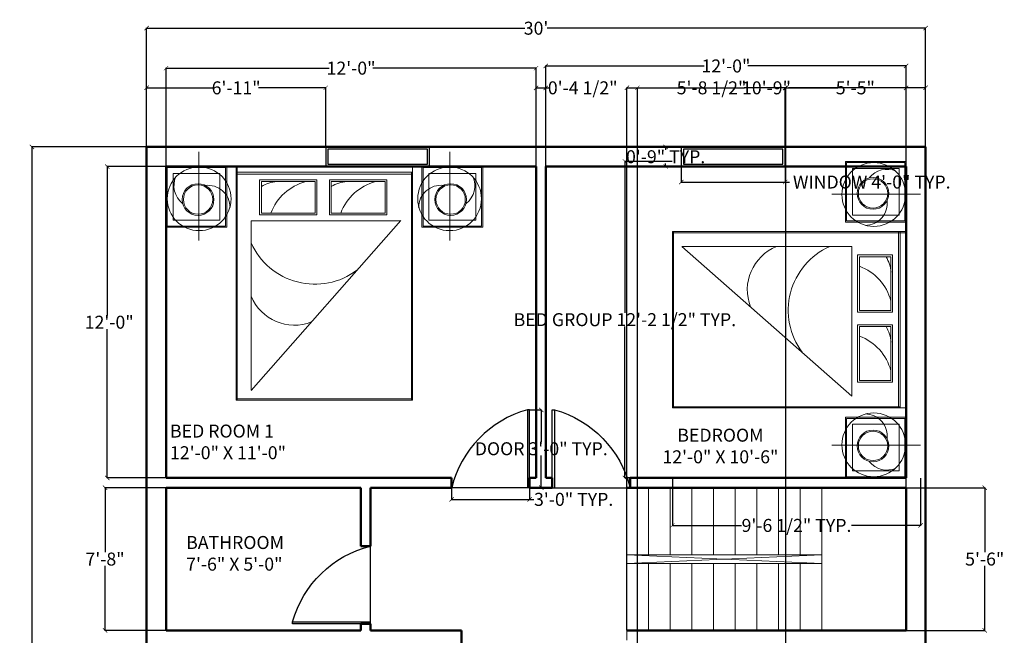
# Model space of a CAD drawing. Units: inches. Extents: x -40 to 418, y 1212 to 1787.
# Tile 3 of 3: x -40 to 415, y 1503 to 1787. Entities that reach past the tile are written whole.
import ezdxf

# ---------------------------------------------------------------- set-up
doc = ezdxf.new("R2010")
doc.units = ezdxf.units.IN
doc.header["$MEASUREMENT"] = 0
for name, color, linetype, lineweight in [('A-ANNO-DIMS', 2, 'Continuous', 18), ('A-AREA-IDEN', 7, 'Continuous', 25), ('A-DOOR', 4, 'Continuous', 25), ('A-FLOR-STRS', 7, 'Continuous', 18), ('A-FURN', 8, 'Continuous', 18), ('A-GLAZ', 4, 'Continuous', 25), ('A-WALL', 7, 'Continuous', 50)]:
    doc.layers.add(name, color=color, linetype=linetype, lineweight=lineweight)
doc.styles.get("Standard").update_dxf_attribs({"font": 'arial.ttf'})
doc.dimstyles.get("Standard").update_dxf_attribs({"dimtxt": 6, "dimasz": 2, "dimexe": 0.18, "dimexo": 0.0625, "dimgap": 0.09, "dimtad": 0, "dimtih": 1, "dimtoh": 1, "dimdec": 0, "dimzin": 0, "dimdsep": 46, "dimlunit": 4, "dimtxsty": 'Standard', "dimblk": 'ARCHTICK', "dimcen": 0.09, "dimadec": 0, "dimazin": 0, "dimtfac": 1, "dimtdec": 0, "dimtofl": 0, "dimtmove": 0, "dimatfit": 3, "dimldrblk": 'ARCHTICK', "dimfxl": 1, "dimtolj": 1, "dimtzin": 0, "dimarcsym": 0})

# ---------------------------------------------------------------- blocks, each defined once
blk = doc.blocks.new('_ArchTick')
at = {"color": 0, "linetype": 'ByBlock', "const_width": 0.15}
blk.add_lwpolyline([(-0.5, -0.5), (0.5, 0.5)], dxfattribs=at)
blk = doc.blocks.new('*D2')
at = {"layer": 'A-ANNO-DIMS', "color": 0, "lineweight": -2, "transparency": 16777216}
for p, q in [((27.43, 1719.7), (27.43, 1765.27)), ((27.43, 1765.09), (102.82, 1765.09)), ((198.43, 1765.09), (123.05, 1765.09)), ((198.43, 1719.7), (198.43, 1765.27))]:
    blk.add_line(p, q, dxfattribs=at)
at = {"layer": 'Defpoints', "color": 0, "transparency": 16777216}
for p in [(198.43, 1765.09), (27.43, 1719.64), (198.43, 1719.64)]:
    blk.add_point(p, dxfattribs=at)
at = {"layer": 'A-ANNO-DIMS', "color": 0, "lineweight": -2, "transparency": 16777216, "xscale": 2, "yscale": 2, "zscale": 2, "rotation": 180}
blk.add_blockref('_ArchTick', (27.43, 1765.09), dxfattribs=at)
at = {"layer": 'A-ANNO-DIMS', "color": 0, "lineweight": -2, "transparency": 16777216, "xscale": 2, "yscale": 2, "zscale": 2}
blk.add_blockref('_ArchTick', (198.43, 1765.09), dxfattribs=at)
at = {"layer": 'A-ANNO-DIMS', "color": 0, "transparency": 16777216, "insert": (112.93, 1765.09), "char_height": 6, "attachment_point": 5}
blk.add_mtext('\\A1;12\'-0"', dxfattribs=at)
blk = doc.blocks.new('*D3')
at = {"layer": 'A-ANNO-DIMS', "color": 0, "lineweight": -2, "transparency": 16777216}
for p, q in [((202.93, 1719.7), (202.93, 1766.27)), ((202.93, 1766.09), (276.07, 1766.09)), ((369.43, 1766.09), (296.3, 1766.09)), ((369.43, 1719.7), (369.43, 1766.27))]:
    blk.add_line(p, q, dxfattribs=at)
at = {"layer": 'Defpoints', "color": 0, "transparency": 16777216}
for p in [(369.43, 1766.09), (202.93, 1719.64), (369.43, 1719.64)]:
    blk.add_point(p, dxfattribs=at)
at = {"layer": 'A-ANNO-DIMS', "color": 0, "lineweight": -2, "transparency": 16777216, "xscale": 2, "yscale": 2, "zscale": 2, "rotation": 180}
blk.add_blockref('_ArchTick', (202.93, 1766.09), dxfattribs=at)
at = {"layer": 'A-ANNO-DIMS', "color": 0, "lineweight": -2, "transparency": 16777216, "xscale": 2, "yscale": 2, "zscale": 2}
blk.add_blockref('_ArchTick', (369.43, 1766.09), dxfattribs=at)
at = {"layer": 'A-ANNO-DIMS', "color": 0, "transparency": 16777216, "insert": (286.18, 1766.09), "char_height": 6, "attachment_point": 5}
blk.add_mtext('\\A1;12\'-0"', dxfattribs=at)
blk = doc.blocks.new('*D4')
at = {"layer": 'A-ANNO-DIMS', "color": 0, "lineweight": -2, "transparency": 16777216}
for p, q in [((18.43, 1728.7), (18.43, 1783.74)), ((378.43, 1728.7), (378.43, 1783.74)), ((18.43, 1783.56), (193.26, 1783.56)), ((378.43, 1783.56), (203.61, 1783.56))]:
    blk.add_line(p, q, dxfattribs=at)
at = {"layer": 'Defpoints', "color": 0, "transparency": 16777216}
for p in [(378.43, 1783.56), (18.43, 1728.64), (378.43, 1728.64)]:
    blk.add_point(p, dxfattribs=at)
at = {"layer": 'A-ANNO-DIMS', "color": 0, "lineweight": -2, "transparency": 16777216, "xscale": 2, "yscale": 2, "zscale": 2, "rotation": 180}
blk.add_blockref('_ArchTick', (18.43, 1783.56), dxfattribs=at)
at = {"layer": 'A-ANNO-DIMS', "color": 0, "lineweight": -2, "transparency": 16777216, "xscale": 2, "yscale": 2, "zscale": 2}
blk.add_blockref('_ArchTick', (378.43, 1783.56), dxfattribs=at)
at = {"layer": 'A-ANNO-DIMS', "color": 0, "transparency": 16777216, "insert": (198.43, 1783.56), "char_height": 6, "attachment_point": 5}
blk.add_mtext("\\A1;30'", dxfattribs=at)
blk = doc.blocks.new('*D5')
at = {"layer": 'A-ANNO-DIMS', "color": 0, "lineweight": -2, "transparency": 16777216}
for p, q in [((18.37, 1728.64), (-34.7, 1728.64)), ((-34.52, 1728.64), (-34.52, 1491.79)), ((-34.52, 1248.64), (-34.52, 1485.48)), ((18.37, 1248.64), (-34.7, 1248.64))]:
    blk.add_line(p, q, dxfattribs=at)
at = {"layer": 'Defpoints', "color": 0, "transparency": 16777216}
for p in [(-34.52, 1728.64), (18.43, 1728.64), (18.43, 1248.64)]:
    blk.add_point(p, dxfattribs=at)
at = {"layer": 'A-ANNO-DIMS', "color": 0, "lineweight": -2, "transparency": 16777216, "xscale": 2, "yscale": 2, "zscale": 2}
for p, rotation in [((-34.52, 1728.64), 90), ((-34.52, 1248.64), 270)]:
    blk.add_blockref('_ArchTick', p, dxfattribs=dict(at, rotation=rotation))
at = {"layer": 'A-ANNO-DIMS', "color": 0, "transparency": 16777216, "insert": (-34.52, 1488.64), "char_height": 6, "attachment_point": 5}
blk.add_mtext("\\A1;40'", dxfattribs=at)
blk = doc.blocks.new('*D6')
at = {"layer": 'A-ANNO-DIMS', "color": 0, "lineweight": -2, "transparency": 16777216}
for p, q in [((27.37, 1719.64), (0.07, 1719.64)), ((0.25, 1719.64), (0.25, 1650.79)), ((0.25, 1575.64), (0.25, 1644.48)), ((27.37, 1575.64), (0.07, 1575.64))]:
    blk.add_line(p, q, dxfattribs=at)
at = {"layer": 'Defpoints', "color": 0, "transparency": 16777216}
for p in [(0.25, 1719.64), (27.43, 1719.64), (27.43, 1575.64)]:
    blk.add_point(p, dxfattribs=at)
at = {"layer": 'A-ANNO-DIMS', "color": 0, "lineweight": -2, "transparency": 16777216, "xscale": 2, "yscale": 2, "zscale": 2}
for p, rotation in [((0.25, 1719.64), 90), ((0.25, 1575.64), 270)]:
    blk.add_blockref('_ArchTick', p, dxfattribs=dict(at, rotation=rotation))
at = {"layer": 'A-ANNO-DIMS', "color": 0, "transparency": 16777216, "insert": (0.25, 1647.64), "char_height": 6, "attachment_point": 5}
blk.add_mtext('\\A1; 12\'-0"', dxfattribs=at)
blk = doc.blocks.new('*D7')
at = {"layer": 'A-ANNO-DIMS', "color": 0, "lineweight": -2, "transparency": 16777216}
for p, q in [((27.37, 1571.14), (-0.93, 1571.14)), ((-0.75, 1571.14), (-0.75, 1541.29)), ((-0.75, 1505.14), (-0.75, 1534.98)), ((27.37, 1505.14), (-0.93, 1505.14))]:
    blk.add_line(p, q, dxfattribs=at)
at = {"layer": 'Defpoints', "color": 0, "transparency": 16777216}
for p in [(-0.75, 1571.14), (27.43, 1571.14), (27.43, 1505.14)]:
    blk.add_point(p, dxfattribs=at)
at = {"layer": 'A-ANNO-DIMS', "color": 0, "lineweight": -2, "transparency": 16777216, "xscale": 2, "yscale": 2, "zscale": 2}
for p, rotation in [((-0.75, 1571.14), 90), ((-0.75, 1505.14), 270)]:
    blk.add_blockref('_ArchTick', p, dxfattribs=dict(at, rotation=rotation))
at = {"layer": 'A-ANNO-DIMS', "color": 0, "transparency": 16777216, "insert": (-0.75, 1538.14), "char_height": 6, "attachment_point": 5}
blk.add_mtext('\\A1;7\'-8"', dxfattribs=at)
blk = doc.blocks.new('DESDFGHJUI')
for p, q in [((-198.91, 1688.99), (-198.91, 1729.95)), ((-82.83, 1688.99), (-82.83, 1729.95)), ((-214.04, 1695.16), (-214.04, 1723.24)), ((-214.04, 1723.24), (-185.96, 1723.24)), ((-213.5, 1695.7), (-213.5, 1722.7)), ((-213.5, 1722.7), (-186.5, 1722.7)), ((-210.8, 1698.4), (-210.8, 1720)), ((-210.8, 1720), (-189.2, 1720)), ((-189.2, 1720), (-189.2, 1698.4)), ((-186.5, 1722.7), (-186.5, 1695.7)), ((-185.96, 1723.24), (-185.96, 1695.16)), ((-181.64, 1723.24), (-181.64, 1615.24)), ((-181.64, 1723.24), (-100.1, 1723.24)), ((-181.64, 1720.54), (-100.1, 1720.54)), ((-181.1, 1723.24), (-181.1, 1615.24)), ((-100.64, 1720.54), (-100.64, 1615.24)), ((-100.1, 1723.24), (-100.1, 1615.24)), ((-67.7, 1723.24), (-95.78, 1723.24)), ((-95.78, 1723.24), (-95.78, 1695.16)), ((-68.24, 1722.7), (-95.24, 1722.7)), ((-95.24, 1722.7), (-95.24, 1695.7)), ((-70.94, 1720), (-92.54, 1720)), ((-92.54, 1720), (-92.54, 1698.4)), ((-70.94, 1698.4), (-70.94, 1720)), ((-68.24, 1695.7), (-68.24, 1722.7)), ((-67.7, 1695.16), (-67.7, 1723.24)), ((-181.64, 1719.73), (-100.1, 1719.73)), ((-170.78, 1700.83), (-170.78, 1717.03)), ((-170.78, 1717.03), (-144.32, 1717.03)), ((-169.97, 1701.64), (-169.97, 1716.22)), ((-169.97, 1716.22), (-145.13, 1716.22)), ((-145.13, 1716.22), (-145.13, 1701.64)), ((-144.32, 1717.03), (-144.32, 1700.83)), ((-138.48, 1700.83), (-138.48, 1717.03)), ((-138.48, 1717.03), (-112.02, 1717.03)), ((-137.67, 1701.64), (-137.67, 1716.22)), ((-137.67, 1716.22), (-112.83, 1716.22)), ((-112.83, 1716.22), (-112.83, 1701.64)), ((-112.02, 1717.03), (-112.02, 1700.83)), ((-189.2, 1698.4), (-210.8, 1698.4)), ((-174.68, 1619.61), (-105.47, 1698.21)), ((-174.64, 1619.8), (-174.64, 1698.13)), ((-174.64, 1698.13), (-105.54, 1698.13)), ((-170.78, 1700.83), (-144.32, 1700.83)), ((-169.97, 1701.64), (-145.13, 1701.64)), ((-138.48, 1700.83), (-112.02, 1700.83)), ((-137.67, 1701.64), (-112.83, 1701.64)), ((-92.54, 1698.4), (-70.94, 1698.4)), ((-185.96, 1695.16), (-214.04, 1695.16)), ((-186.5, 1695.7), (-213.5, 1695.7)), ((-95.78, 1695.16), (-67.7, 1695.16)), ((-95.24, 1695.7), (-68.24, 1695.7)), ((-131.52, 1615.74), (-181.64, 1615.74)), ((-100.1, 1615.78), (-175.16, 1615.78)), ((-100.1, 1615.24), (-181.64, 1615.24))]:
    blk.add_line(p, q)
for centre, radius in [((-198.74, 1708.29), 14.73), ((-83.01, 1708.29), 14.73), ((-199.23, 1707.96), 7.32), ((-199.23, 1707.96), 6.78), ((-82.52, 1707.96), 7.32), ((-82.52, 1707.96), 6.78)]:
    blk.add_circle(centre, radius)
for centre, radius, start, end in [((-200.04, 1714.33), 10.36, 155.9567, 231.7564), ((-161.57, 1700.2), 16.13, 94.4656, 121.4122), ((-143.54, 1693.44), 23.54, 104.6626, 159.6122), ((-129.26, 1700.2), 16.13, 94.4656, 121.4122), ((-111.24, 1693.44), 23.54, 104.6626, 159.6122), ((-81.71, 1714.33), 10.36, 308.2436, 24.0433), ((-194.74, 1704.25), 10.3, 0.4104, 96.764), ((-87.01, 1704.25), 10.3, 83.236, 179.5896), ((-145.2, 1701.08), 32.28, 204.0563, 306.8492), ((-154.7, 1671.44), 21.57, 202.1275, 291.5505)]:
    blk.add_arc(centre, radius, start, end)
blk = doc.blocks.new('EREGTHYGUI')
for p, q in [((195.43, 1607.14), (194.43, 1607.14)), ((194.43, 1607.14), (194.43, 1571.14)), ((195.43, 1571.14), (195.43, 1607.14)), ((195.43, 1571.14), (159.43, 1571.14))]:
    blk.add_line(p, q)
blk.add_arc((207.79, 1559.14), 49.82, 105.5486, 166.0653)
blk = doc.blocks.new('WIN-48IN')
for points in [[(0, 0), (9, 0), (9, 48), (0, 48)], [(1, 1), (8, 1), (8, 47), (1, 47)]]:
    blk.add_lwpolyline(points, close=True)
blk = doc.blocks.new('*D17')
at = {"layer": 'A-ANNO-DIMS', "color": 0, "lineweight": -2, "transparency": 16777216}
for p, q in [((195.5, 1607.14), (201.01, 1607.14)), ((200.83, 1607.14), (200.83, 1592.33)), ((200.83, 1571.14), (200.83, 1585.94)), ((195.5, 1571.14), (201.01, 1571.14))]:
    blk.add_line(p, q, dxfattribs=at)
at = {"layer": 'Defpoints', "color": 0, "transparency": 16777216}
for p in [(195.43, 1607.14), (200.83, 1607.14), (195.43, 1571.14)]:
    blk.add_point(p, dxfattribs=at)
at = {"layer": 'A-ANNO-DIMS', "color": 0, "lineweight": -2, "transparency": 16777216, "xscale": 2, "yscale": 2, "zscale": 2}
for p, rotation in [((200.83, 1607.14), 90), ((200.83, 1571.14), 270)]:
    blk.add_blockref('_ArchTick', p, dxfattribs=dict(at, rotation=rotation))
at = {"layer": 'A-ANNO-DIMS', "color": 0, "transparency": 16777216, "insert": (200.83, 1589.14), "char_height": 6, "attachment_point": 5}
blk.add_mtext('\\A1;DOOR 3\'-0" TYP.', dxfattribs=at)
blk = doc.blocks.new('*D18')
at = {"layer": 'A-ANNO-DIMS', "color": 0, "lineweight": -2, "transparency": 16777216}
for p, q in [((159.43, 1571.07), (159.43, 1565.56)), ((195.43, 1571.07), (195.43, 1565.56)), ((159.43, 1565.74), (195.43, 1565.74)), ((195.43, 1565.74), (197.43, 1565.74))]:
    blk.add_line(p, q, dxfattribs=at)
at = {"layer": 'Defpoints', "color": 0, "transparency": 16777216}
for p in [(159.43, 1571.14), (195.43, 1571.14), (195.43, 1565.74)]:
    blk.add_point(p, dxfattribs=at)
at = {"layer": 'A-ANNO-DIMS', "color": 0, "lineweight": -2, "transparency": 16777216, "xscale": 2, "yscale": 2, "zscale": 2, "rotation": 180}
blk.add_blockref('_ArchTick', (159.43, 1565.74), dxfattribs=at)
at = {"layer": 'A-ANNO-DIMS', "color": 0, "lineweight": -2, "transparency": 16777216, "xscale": 2, "yscale": 2, "zscale": 2}
blk.add_blockref('_ArchTick', (195.43, 1565.74), dxfattribs=at)
at = {"layer": 'A-ANNO-DIMS', "color": 0, "transparency": 16777216, "insert": (215.81, 1565.74), "char_height": 6, "attachment_point": 5}
blk.add_mtext('\\A1;3\'-0" TYP.', dxfattribs=at)
blk = doc.blocks.new('*D19')
at = {"layer": 'A-ANNO-DIMS', "color": 0, "lineweight": -2, "transparency": 16777216}
for p, q in [((265.52, 1719.57), (265.52, 1712.26)), ((313.52, 1719.57), (313.52, 1712.26)), ((265.52, 1712.44), (313.52, 1712.44)), ((313.52, 1712.44), (315.52, 1712.44))]:
    blk.add_line(p, q, dxfattribs=at)
at = {"layer": 'Defpoints', "color": 0, "transparency": 16777216}
for p in [(265.52, 1719.64), (313.52, 1719.64), (313.52, 1712.44)]:
    blk.add_point(p, dxfattribs=at)
at = {"layer": 'A-ANNO-DIMS', "color": 0, "lineweight": -2, "transparency": 16777216, "xscale": 2, "yscale": 2, "zscale": 2, "rotation": 180}
blk.add_blockref('_ArchTick', (265.52, 1712.44), dxfattribs=at)
at = {"layer": 'A-ANNO-DIMS', "color": 0, "lineweight": -2, "transparency": 16777216, "xscale": 2, "yscale": 2, "zscale": 2}
blk.add_blockref('_ArchTick', (313.52, 1712.44), dxfattribs=at)
at = {"layer": 'A-ANNO-DIMS', "color": 0, "transparency": 16777216, "insert": (353.57, 1712.44), "char_height": 6, "attachment_point": 5}
blk.add_mtext('\\A1;WINDOW 4\'-0" TYP.', dxfattribs=at)
blk = doc.blocks.new('*D20')
at = {"layer": 'A-ANNO-DIMS', "color": 0, "lineweight": -2, "transparency": 16777216}
for p, q in [((265.46, 1728.64), (258.14, 1728.64)), ((258.32, 1728.64), (258.32, 1727.29)), ((258.32, 1719.64), (258.32, 1720.98)), ((265.46, 1719.64), (258.14, 1719.64))]:
    blk.add_line(p, q, dxfattribs=at)
at = {"layer": 'Defpoints', "color": 0, "transparency": 16777216}
for p in [(265.52, 1728.64), (258.32, 1719.64), (265.52, 1719.64)]:
    blk.add_point(p, dxfattribs=at)
at = {"layer": 'A-ANNO-DIMS', "color": 0, "lineweight": -2, "transparency": 16777216, "xscale": 2, "yscale": 2, "zscale": 2}
for p, rotation in [((258.32, 1728.64), 90), ((258.32, 1719.64), 270)]:
    blk.add_blockref('_ArchTick', p, dxfattribs=dict(at, rotation=rotation))
at = {"layer": 'A-ANNO-DIMS', "color": 0, "transparency": 16777216, "insert": (258.32, 1724.14), "char_height": 6, "attachment_point": 5}
blk.add_mtext('\\A1;0\'-9" TYP.', dxfattribs=at)
blk = doc.blocks.new('*D23')
at = {"layer": 'A-ANNO-DIMS', "color": 0, "lineweight": -2, "transparency": 16777216}
for p, q in [((261.37, 1721.98), (239.3, 1721.98)), ((239.48, 1721.98), (239.48, 1652)), ((239.48, 1575.64), (239.48, 1645.61)), ((261.37, 1575.64), (239.3, 1575.64))]:
    blk.add_line(p, q, dxfattribs=at)
at = {"layer": 'Defpoints', "color": 0, "transparency": 16777216}
for p in [(261.43, 1721.98), (239.48, 1575.64), (261.43, 1575.64)]:
    blk.add_point(p, dxfattribs=at)
at = {"layer": 'A-ANNO-DIMS', "color": 0, "lineweight": -2, "transparency": 16777216, "xscale": 2, "yscale": 2, "zscale": 2}
for p, rotation in [((239.48, 1721.98), 90), ((239.48, 1575.64), 270)]:
    blk.add_blockref('_ArchTick', p, dxfattribs=dict(at, rotation=rotation))
at = {"layer": 'A-ANNO-DIMS', "color": 0, "transparency": 16777216, "insert": (239.48, 1648.81), "char_height": 6, "attachment_point": 5}
blk.add_mtext('\\A1;BED GROUP 12\'-2 1/2" TYP.', dxfattribs=at)
blk = doc.blocks.new('*D24')
at = {"layer": 'A-ANNO-DIMS', "color": 0, "lineweight": -2, "transparency": 16777216}
for p, q in [((261.43, 1575.57), (261.43, 1553.51)), ((376.15, 1575.57), (376.15, 1553.51)), ((261.43, 1553.69), (293.42, 1553.69)), ((376.15, 1553.69), (344.16, 1553.69))]:
    blk.add_line(p, q, dxfattribs=at)
at = {"layer": 'Defpoints', "color": 0, "transparency": 16777216}
for p in [(261.43, 1575.64), (376.15, 1575.64), (376.15, 1553.69)]:
    blk.add_point(p, dxfattribs=at)
at = {"layer": 'A-ANNO-DIMS', "color": 0, "lineweight": -2, "transparency": 16777216, "xscale": 2, "yscale": 2, "zscale": 2, "rotation": 180}
blk.add_blockref('_ArchTick', (261.43, 1553.69), dxfattribs=at)
at = {"layer": 'A-ANNO-DIMS', "color": 0, "lineweight": -2, "transparency": 16777216, "xscale": 2, "yscale": 2, "zscale": 2}
blk.add_blockref('_ArchTick', (376.15, 1553.69), dxfattribs=at)
at = {"layer": 'A-ANNO-DIMS', "color": 0, "transparency": 16777216, "insert": (318.79, 1553.69), "char_height": 6, "attachment_point": 5}
blk.add_mtext('\\A1;9\'-6 1/2" TYP.', dxfattribs=at)
blk = doc.blocks.new('*D31')
at = {"layer": 'A-ANNO-DIMS', "color": 0, "lineweight": -2, "transparency": 16777216}
for p, q in [((240.43, 1505.2), (240.43, 1756.17)), ((240.43, 1755.99), (294.82, 1755.99)), ((369.43, 1755.99), (315.05, 1755.99)), ((369.43, 1505.2), (369.43, 1756.17))]:
    blk.add_line(p, q, dxfattribs=at)
at = {"layer": 'Defpoints', "color": 0, "transparency": 16777216}
for p in [(369.43, 1755.99), (240.43, 1505.14), (369.43, 1505.14)]:
    blk.add_point(p, dxfattribs=at)
at = {"layer": 'A-ANNO-DIMS', "color": 0, "lineweight": -2, "transparency": 16777216, "xscale": 2, "yscale": 2, "zscale": 2, "rotation": 180}
blk.add_blockref('_ArchTick', (240.43, 1755.99), dxfattribs=at)
at = {"layer": 'A-ANNO-DIMS', "color": 0, "lineweight": -2, "transparency": 16777216, "xscale": 2, "yscale": 2, "zscale": 2}
blk.add_blockref('_ArchTick', (369.43, 1755.99), dxfattribs=at)
at = {"layer": 'A-ANNO-DIMS', "color": 0, "transparency": 16777216, "insert": (304.93, 1755.99), "char_height": 6, "attachment_point": 5}
blk.add_mtext('\\A1;10\'-9"', dxfattribs=at)
blk = doc.blocks.new('*D32')
at = {"layer": 'A-ANNO-DIMS', "color": 0, "lineweight": -2, "transparency": 16777216}
for p, q in [((369.5, 1571.14), (405.96, 1571.14)), ((405.78, 1571.14), (405.78, 1541.29)), ((405.78, 1505.14), (405.78, 1534.98)), ((369.5, 1505.14), (405.96, 1505.14))]:
    blk.add_line(p, q, dxfattribs=at)
at = {"layer": 'Defpoints', "color": 0, "transparency": 16777216}
for p in [(369.43, 1571.14), (405.78, 1571.14), (369.43, 1505.14)]:
    blk.add_point(p, dxfattribs=at)
at = {"layer": 'A-ANNO-DIMS', "color": 0, "lineweight": -2, "transparency": 16777216, "xscale": 2, "yscale": 2, "zscale": 2}
for p, rotation in [((405.78, 1571.14), 90), ((405.78, 1505.14), 270)]:
    blk.add_blockref('_ArchTick', p, dxfattribs=dict(at, rotation=rotation))
at = {"layer": 'A-ANNO-DIMS', "color": 0, "transparency": 16777216, "insert": (405.78, 1538.14), "char_height": 6, "attachment_point": 5}
blk.add_mtext('\\A1;5\'-6"', dxfattribs=at)
blk = doc.blocks.new('*D36')
at = {"layer": 'A-ANNO-DIMS', "color": 0, "lineweight": -2, "transparency": 16777216}
for p, q in [((18.43, 1728.7), (18.43, 1756.17)), ((18.43, 1755.99), (49.41, 1755.99)), ((101.22, 1755.99), (70.24, 1755.99)), ((101.22, 1728.7), (101.22, 1756.17))]:
    blk.add_line(p, q, dxfattribs=at)
at = {"layer": 'Defpoints', "color": 0, "transparency": 16777216}
for p in [(101.22, 1755.99), (18.43, 1728.64), (101.22, 1728.64)]:
    blk.add_point(p, dxfattribs=at)
at = {"layer": 'A-ANNO-DIMS', "color": 0, "lineweight": -2, "transparency": 16777216, "xscale": 2, "yscale": 2, "zscale": 2, "rotation": 180}
blk.add_blockref('_ArchTick', (18.43, 1755.99), dxfattribs=at)
at = {"layer": 'A-ANNO-DIMS', "color": 0, "lineweight": -2, "transparency": 16777216, "xscale": 2, "yscale": 2, "zscale": 2}
blk.add_blockref('_ArchTick', (101.22, 1755.99), dxfattribs=at)
at = {"layer": 'A-ANNO-DIMS', "color": 0, "transparency": 16777216, "insert": (59.83, 1755.99), "char_height": 6, "attachment_point": 5}
blk.add_mtext('\\A1;6\'-11"', dxfattribs=at)
blk = doc.blocks.new('*D37')
at = {"layer": 'A-ANNO-DIMS', "color": 0, "lineweight": -2, "transparency": 16777216}
for p, q in [((313.52, 1728.7), (313.52, 1756.17)), ((313.52, 1755.99), (337.91, 1755.99)), ((378.43, 1755.99), (354.04, 1755.99)), ((378.43, 1728.7), (378.43, 1756.17))]:
    blk.add_line(p, q, dxfattribs=at)
at = {"layer": 'Defpoints', "color": 0, "transparency": 16777216}
for p in [(378.43, 1755.99), (313.52, 1728.64), (378.43, 1728.64)]:
    blk.add_point(p, dxfattribs=at)
at = {"layer": 'A-ANNO-DIMS', "color": 0, "lineweight": -2, "transparency": 16777216, "xscale": 2, "yscale": 2, "zscale": 2, "rotation": 180}
blk.add_blockref('_ArchTick', (313.52, 1755.99), dxfattribs=at)
at = {"layer": 'A-ANNO-DIMS', "color": 0, "lineweight": -2, "transparency": 16777216, "xscale": 2, "yscale": 2, "zscale": 2}
blk.add_blockref('_ArchTick', (378.43, 1755.99), dxfattribs=at)
at = {"layer": 'A-ANNO-DIMS', "color": 0, "transparency": 16777216, "insert": (345.98, 1755.99), "char_height": 6, "attachment_point": 5}
blk.add_mtext('\\A1;5\'-5"', dxfattribs=at)
blk = doc.blocks.new('*D39')
at = {"layer": 'A-ANNO-DIMS', "color": 0, "lineweight": -2, "transparency": 16777216}
for p, q in [((245.24, 1474.1), (245.24, 1756.17)), ((245.24, 1755.99), (264.49, 1755.99)), ((313.85, 1755.99), (294.6, 1755.99)), ((313.85, 1474.1), (313.85, 1756.17))]:
    blk.add_line(p, q, dxfattribs=at)
at = {"layer": 'Defpoints', "color": 0, "transparency": 16777216}
for p in [(313.85, 1755.99), (245.24, 1474.03), (313.85, 1474.03)]:
    blk.add_point(p, dxfattribs=at)
at = {"layer": 'A-ANNO-DIMS', "color": 0, "lineweight": -2, "transparency": 16777216, "xscale": 2, "yscale": 2, "zscale": 2, "rotation": 180}
blk.add_blockref('_ArchTick', (245.24, 1755.99), dxfattribs=at)
at = {"layer": 'A-ANNO-DIMS', "color": 0, "lineweight": -2, "transparency": 16777216, "xscale": 2, "yscale": 2, "zscale": 2}
blk.add_blockref('_ArchTick', (313.85, 1755.99), dxfattribs=at)
at = {"layer": 'A-ANNO-DIMS', "color": 0, "transparency": 16777216, "insert": (279.54, 1755.99), "char_height": 6, "attachment_point": 5}
blk.add_mtext('\\A1;5\'-8 1/2"', dxfattribs=at)
blk = doc.blocks.new('*D44')
at = {"layer": 'A-ANNO-DIMS', "color": 0, "lineweight": -2, "transparency": 16777216}
for p, q in [((198.43, 1719.7), (198.43, 1756.17)), ((198.43, 1755.99), (202.93, 1755.99)), ((202.93, 1719.7), (202.93, 1756.17)), ((202.93, 1755.99), (204.93, 1755.99))]:
    blk.add_line(p, q, dxfattribs=at)
at = {"layer": 'Defpoints', "color": 0, "transparency": 16777216}
for p in [(202.93, 1755.99), (198.43, 1719.64), (202.93, 1719.64)]:
    blk.add_point(p, dxfattribs=at)
at = {"layer": 'A-ANNO-DIMS', "color": 0, "lineweight": -2, "transparency": 16777216, "xscale": 2, "yscale": 2, "zscale": 2, "rotation": 180}
blk.add_blockref('_ArchTick', (198.43, 1755.99), dxfattribs=at)
at = {"layer": 'A-ANNO-DIMS', "color": 0, "lineweight": -2, "transparency": 16777216, "xscale": 2, "yscale": 2, "zscale": 2}
blk.add_blockref('_ArchTick', (202.93, 1755.99), dxfattribs=at)
at = {"layer": 'A-ANNO-DIMS', "color": 0, "transparency": 16777216, "insert": (219.99, 1755.99), "char_height": 6, "attachment_point": 5}
blk.add_mtext('\\A1;0\'-4 1/2"', dxfattribs=at)

msp = doc.modelspace()

# ---------------------------------------------------------------- linework, layer by layer
at = {"layer": 'A-FLOR-STRS'}
for p, q in [((240.43, 1571.14), (240.43, 1540.14)), ((250.43, 1571.14), (250.43, 1540.14)), ((260.43, 1571.14), (260.43, 1540.14)), ((270.43, 1571.14), (270.43, 1540.14)), ((280.43, 1571.14), (280.43, 1540.14)), ((290.43, 1571.14), (290.43, 1540.14)), ((300.43, 1571.14), (300.43, 1540.14)), ((310.43, 1571.14), (310.43, 1540.14)), ((320.43, 1571.14), (320.43, 1540.14)), ((330.43, 1571.14), (330.43, 1505.14)), ((330.43, 1540.14), (240.43, 1540.14)), ((240.43, 1536.14), (330.43, 1540.14)), ((240.43, 1540.14), (330.43, 1536.14)), ((330.43, 1536.14), (240.43, 1536.14)), ((240.43, 1536.14), (240.43, 1500.64)), ((250.43, 1536.14), (250.43, 1505.14)), ((260.43, 1536.14), (260.43, 1505.14)), ((270.43, 1536.14), (270.43, 1505.14)), ((280.43, 1536.14), (280.43, 1505.14)), ((290.43, 1536.14), (290.43, 1505.14)), ((300.43, 1536.14), (300.43, 1505.14)), ((310.43, 1536.14), (310.43, 1505.14)), ((320.43, 1536.14), (320.43, 1505.14))]:
    msp.add_line(p, q, dxfattribs=at)
at = {"layer": 'A-WALL'}
for p, q in [((18.43, 1728.64), (378.43, 1728.64)), ((18.43, 1248.64), (18.43, 1728.64)), ((378.43, 1728.64), (378.43, 1248.64)), ((27.43, 1719.64), (198.43, 1719.64)), ((27.43, 1575.64), (27.43, 1719.64)), ((198.43, 1719.64), (198.43, 1575.64)), ((202.93, 1719.64), (202.93, 1575.64)), ((202.93, 1719.64), (369.43, 1719.64)), ((369.43, 1719.64), (369.43, 1575.64)), ((27.43, 1575.64), (159.43, 1575.64)), ((159.43, 1575.64), (159.43, 1571.14)), ((195.43, 1575.64), (195.43, 1571.14)), ((195.43, 1575.64), (198.43, 1575.64)), ((202.93, 1575.64), (205.93, 1575.64)), ((205.93, 1575.64), (205.93, 1571.14)), ((241.93, 1575.64), (241.93, 1571.14)), ((241.93, 1575.64), (369.43, 1575.64)), ((27.43, 1571.14), (117.43, 1571.14)), ((27.43, 1505.14), (27.43, 1571.14)), ((117.43, 1544.14), (117.43, 1571.14)), ((121.93, 1571.14), (159.43, 1571.14)), ((121.93, 1544.14), (121.93, 1571.14)), ((195.43, 1571.14), (205.93, 1571.14)), ((240.43, 1571.14), (369.43, 1571.14)), ((369.43, 1571.14), (369.43, 1505.14)), ((117.43, 1544.14), (121.93, 1544.14)), ((117.43, 1505.14), (117.43, 1508.14)), ((117.43, 1508.14), (121.93, 1508.14)), ((121.93, 1505.14), (121.93, 1508.14)), ((27.43, 1505.14), (117.43, 1505.14)), ((121.93, 1505.14), (163.93, 1505.14)), ((163.93, 1443.64), (163.93, 1505.14)), ((240.43, 1505.14), (369.43, 1505.14))]:
    msp.add_line(p, q, dxfattribs=at)

# ---------------------------------------------------------------- block references
at = {"layer": 'A-DOOR'}
msp.add_blockref('EREGTHYGUI', (0, 0), dxfattribs=at)
at = {"layer": 'A-DOOR', "xscale": -1}
msp.add_blockref('EREGTHYGUI', (401.37, 0), dxfattribs=at)
at = {"layer": 'A-DOOR', "xscale": -1, "rotation": 90}
msp.add_blockref('EREGTHYGUI', (1693.07, 1703.57), dxfattribs=at)
at = {"layer": 'A-FURN'}
msp.add_blockref('DESDFGHJUI', (241.48, -3.6), dxfattribs=at)
at = {"layer": 'A-FURN', "rotation": 270}
msp.add_blockref('DESDFGHJUI', (-1353.8, 1507.93), dxfattribs=at)
at = {"layer": 'A-GLAZ', "rotation": 269.9999999999995}
for p in [(101.22, 1728.64), (265.52, 1728.64)]:
    msp.add_blockref('WIN-48IN', p, dxfattribs=at)

# ---------------------------------------------------------------- texts
at = {"layer": 'A-AREA-IDEN', "char_height": 6, "attachment_point": 1}
for s, width, insert in [(' BED ROOM 1\\P 12\'-0" X 11\'-0"', 120.8402, (27.43, 1600.31)), ('\\pxqc;BEDROOM\\P12\'-0" X 10\'-6"', 74.3114, (246.48, 1598.41)), ('BATHROOM\\P7\'-6" X 5\'-0"', 215.4125, (36.73, 1548.79))]:
    msp.add_mtext_dynamic_manual_height_columns(s, width=width, gutter_width=30, heights=[0], dxfattribs=dict(at, insert=insert))

# ---------------------------------------------------------------- dimensions: what is measured, and where the dimension line sits
at = {"layer": 'A-ANNO-DIMS'}
for base, p1, p2, override, picture, middle in [((378.43, 1783.56), (18.43, 1728.64), (378.43, 1728.64), {"dimclrd": 0, "dimclre": 0, "dimclrt": 0}, '*D4', (198.43, 1783.56)), ((202.93, 1755.99), (198.43, 1719.64), (202.93, 1719.64), {"dimdec": 1, "dimlfac": 1, "dimrnd": 0, "dimzin": 1, "dimdsep": 46, "dimlunit": 4, "dimfrac": 2}, '*D44', (219.99, 1755.99)), ((313.85, 1755.99), (245.24, 1474.03), (313.85, 1474.03), {"dimdec": 1, "dimlfac": 1, "dimrnd": 0, "dimzin": 1, "dimdsep": 46, "dimlunit": 4, "dimfrac": 2}, '*D39', (279.54, 1755.99)), ((101.22, 1755.99), (18.43, 1728.64), (101.22, 1728.64), {"dimdec": 1, "dimlfac": 1, "dimrnd": 0, "dimzin": 1, "dimdsep": 46, "dimlunit": 4, "dimfrac": 2}, '*D36', (59.83, 1755.99)), ((369.43, 1755.99), (240.43, 1505.14), (369.43, 1505.14), {"dimdec": 1, "dimlfac": 1, "dimrnd": 0, "dimzin": 1, "dimdsep": 46, "dimlunit": 4, "dimfrac": 2}, '*D31', (304.93, 1755.99)), ((378.43, 1755.99), (313.52, 1728.64), (378.43, 1728.64), {"dimdec": 1, "dimlfac": 1, "dimrnd": 0, "dimzin": 1, "dimdsep": 46, "dimlunit": 4, "dimfrac": 2}, '*D37', (345.98, 1755.99))]:
    dim = msp.add_linear_dim(base=base, p1=p1, p2=p2, dimstyle='Standard', override=override, dxfattribs=at)
    dim.commit()
    dim.dimension.update_dxf_attribs({"geometry": picture, "text_midpoint": middle})
for base, p1, p2, text, override, picture, middle in [((198.43, 1765.09), (27.43, 1719.64), (198.43, 1719.64), '12\'-0"', {"dimclrd": 0, "dimclre": 0, "dimclrt": 0}, '*D2', (112.93, 1765.09)), ((369.43, 1766.09), (202.93, 1719.64), (369.43, 1719.64), '12\'-0"', {"dimclrd": 0, "dimclre": 0, "dimclrt": 0}, '*D3', (286.18, 1766.09)), ((313.52, 1712.44), (265.52, 1719.64), (313.52, 1719.64), 'WINDOW <> TYP.', {"dimdec": 1, "dimlfac": 1, "dimrnd": 0, "dimzin": 1, "dimdsep": 46, "dimlunit": 4, "dimfrac": 2}, '*D19', (353.57, 1712.44)), ((195.43, 1565.74), (159.43, 1571.14), (195.43, 1571.14), '<> TYP.', {"dimdec": 1, "dimlfac": 1, "dimrnd": 0, "dimzin": 1, "dimdsep": 46, "dimlunit": 4, "dimfrac": 2}, '*D18', (215.81, 1565.74)), ((376.15, 1553.69), (261.43, 1575.64), (376.15, 1575.64), '<> TYP.', {"dimdec": 1, "dimlfac": 1, "dimrnd": 0, "dimzin": 1, "dimdsep": 46, "dimlunit": 4, "dimfrac": 2}, '*D24', (318.79, 1553.69))]:
    dim = msp.add_linear_dim(base=base, p1=p1, p2=p2, text=text, dimstyle='Standard', override=override, dxfattribs=at)
    dim.commit()
    dim.dimension.update_dxf_attribs({"geometry": picture, "text_midpoint": middle})
for base, p1, p2, override, picture, middle in [((-34.52, 1728.64), (18.43, 1248.64), (18.43, 1728.64), {"dimclrd": 0, "dimclre": 0, "dimclrt": 0}, '*D5', (-34.52, 1488.64)), ((405.78, 1571.14), (369.43, 1505.14), (369.43, 1571.14), {"dimdec": 1, "dimlfac": 1, "dimrnd": 0, "dimzin": 1, "dimdsep": 46, "dimlunit": 4, "dimfrac": 2}, '*D32', (405.78, 1538.14))]:
    dim = msp.add_linear_dim(base=base, p1=p1, p2=p2, angle=90, dimstyle='Standard', override=override, dxfattribs=at)
    dim.commit()
    dim.dimension.update_dxf_attribs({"geometry": picture, "text_midpoint": middle})
for base, p1, p2, angle, text, override, picture, middle in [((258.32, 1719.64), (265.52, 1728.64), (265.52, 1719.64), 270, '<> TYP.', {"dimdec": 1, "dimlfac": 1, "dimrnd": 0, "dimzin": 1, "dimdsep": 46, "dimlunit": 4, "dimfrac": 2}, '*D20', (258.32, 1724.14)), ((0.25, 1719.64), (27.43, 1575.64), (27.43, 1719.64), 90, ' 12\'-0"', {"dimclrd": 0, "dimclre": 0, "dimclrt": 0}, '*D6', (0.25, 1647.64)), ((239.48, 1575.64), (261.43, 1721.98), (261.43, 1575.64), 270, 'BED GROUP <> TYP.', {"dimdec": 1, "dimlfac": 1, "dimrnd": 0, "dimzin": 1, "dimdsep": 46, "dimlunit": 4, "dimfrac": 2}, '*D23', (239.48, 1648.81)), ((200.83, 1607.14), (195.43, 1571.14), (195.43, 1607.14), 90, 'DOOR <> TYP.', {"dimdec": 1, "dimlfac": 1, "dimrnd": 0, "dimzin": 1, "dimdsep": 46, "dimlunit": 4, "dimfrac": 2}, '*D17', (200.83, 1589.14)), ((-0.75, 1571.14), (27.43, 1505.14), (27.43, 1571.14), 90, '7\'-8"', {"dimclrd": 0, "dimclre": 0, "dimclrt": 0}, '*D7', (-0.75, 1538.14))]:
    dim = msp.add_linear_dim(base=base, p1=p1, p2=p2, angle=angle, text=text, dimstyle='Standard', override=override, dxfattribs=at)
    dim.commit()
    dim.dimension.update_dxf_attribs({"geometry": picture, "text_midpoint": middle})

doc.saveas('drawing.dxf')
